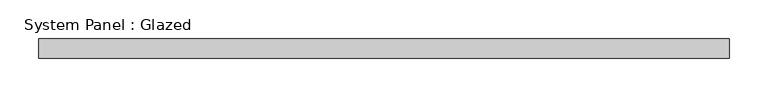
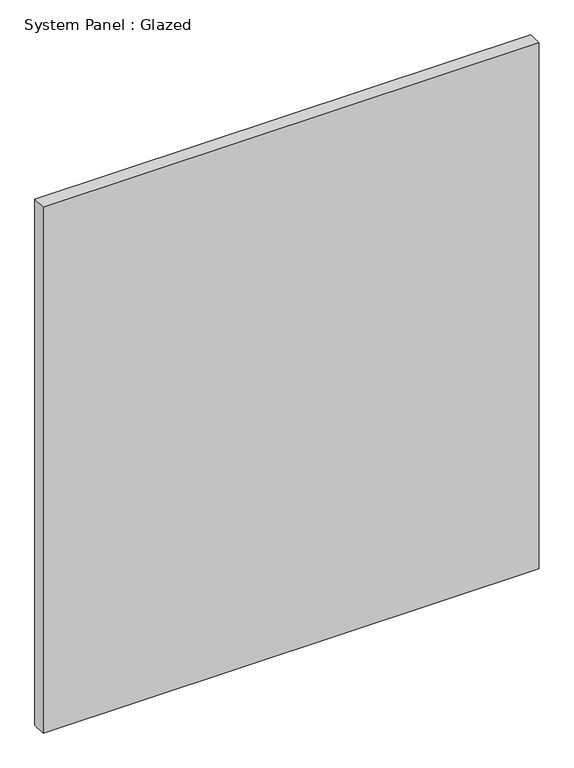
"""IFC4 building model written with IfcOpenShell, lengths in millimetres: plate geometry, System Panel : Glazed."""

from ifc_helpers import new_model, si_unit, origin, origin_with_axes, place, context, project, spatial, polyline, outline, extrude, source, transform, mapped, element, save


def system_panel_glazed_b791fe2b(model_context):
    return source(origin(), model_context, "Body", "SweptSolid", [
        extrude(outline(polyline([(447.675, 19.05), (-447.675, 19.05), (-447.675, 44.45), (447.675, 44.45), (447.675, 19.05)])), origin_with_axes(), (0.0, 0.0, 1.0), 1003.3),
    ])


if __name__ == "__main__":
    model = new_model("IFC4")
    model_context = context("Model", 3, world=origin())
    ifc_project = project(units=[si_unit("LENGTHUNIT", "METRE", prefix="MILLI")], contexts=[model_context])
    site = spatial("IfcSite", under=ifc_project)
    building = spatial("IfcBuilding", under=site)
    placement = place(None, origin())
    system_panel_glazed_shape = system_panel_glazed_b791fe2b(model_context)
    element("IfcPlate", 1, ObjectType="System Panel : Glazed", at=placement, inside=building, context=model_context, shape_type="MappedRepresentation", body=[
        mapped(system_panel_glazed_shape, transform((0.0, 0.0, 0.0), x_axis=(1.0, 0.0, 0.0), y_axis=(0.0, 1.0, 0.0), z_axis=(0.0, 0.0, 1.0))),
    ])
    save(model, "model.ifc")

# Revit data of these elements
# Type "System Panel : Glazed"
#   Construction Type Id = "GSP4R"
#   Analytic Construction = "1/8 in Pilkington single glazing"
#   Visual Light Transmittance = 0.9
#   Solar Heat Gain Coefficient = 0.86
#   Heat Transfer Coefficient (U) = 1.18115 BTU/(h·ft²·°F)
#   Define Thermal Properties by = 1
# Element 1 (IfcPlate, "System Panel : Glazed")
#   Materials on its faces: "Glass"
# Materials
#   "Glass": class "Glass", colour RGB 0 128 192, transparency 0.75, Description = "Soda Lime Glass", Cost = 0
